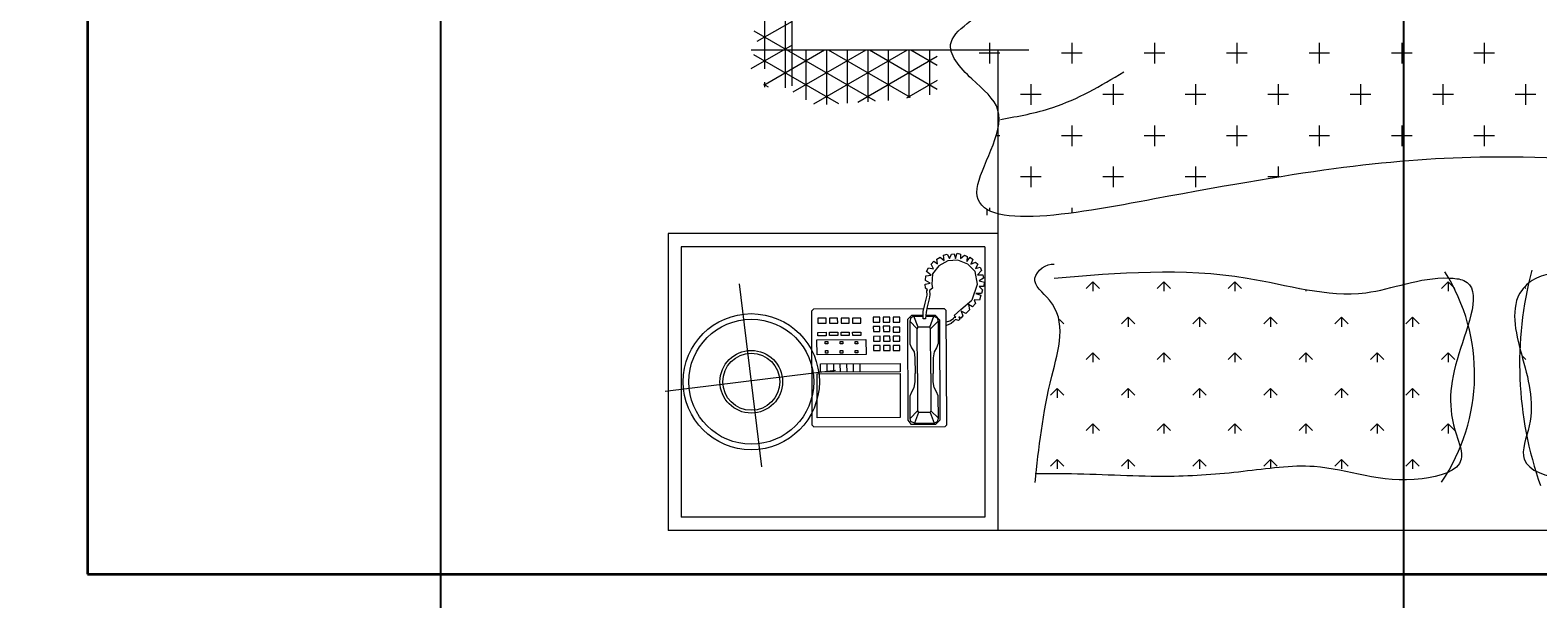
# Model space of a CAD drawing. Units: inches. Extents: x 3731 to 4318, y 1310 to 2388.
# Tile 9 of 57: x 3944 to 4038, y 1363 to 1398. Entities that reach past the tile are written whole.
import ezdxf

# ---------------------------------------------------------------- set-up
doc = ezdxf.new("R2010")
doc.units = ezdxf.units.IN
for name, color, linetype, lineweight in [('A-ANNO-DIMS', 2, 'Continuous', 18), ('A-FURN', 8, 'Continuous', 13), ('A-WALL', 7, 'Continuous', 35)]:
    doc.layers.add(name, color=color, linetype=linetype, lineweight=lineweight)
doc.styles.get("Standard").update_dxf_attribs({"font": 'arial.ttf'})
doc.dimstyles.get("Standard").update_dxf_attribs({"dimtxt": 0.18, "dimasz": 0.18, "dimexe": 0.18, "dimexo": 0.0625, "dimgap": 0.09, "dimtad": 0, "dimtih": 1, "dimtoh": 1, "dimdec": 4, "dimzin": 0, "dimdsep": 46, "dimtxsty": 'Standard', "dimcen": 0.09, "dimadec": 0, "dimazin": 0, "dimtfac": 1, "dimtdec": 4, "dimtofl": 0, "dimtmove": 0, "dimatfit": 3, "dimfxl": 1, "dimtolj": 1, "dimtzin": 0, "dimarcsym": 0})

# ---------------------------------------------------------------- blocks, each defined once
blk = doc.blocks.new('A$C200C7901')
for p, q in [((0.5, 2.3334), (2, 2.3334)), ((2, 2.3334), (2.5, 2.3334)), ((2, 1.6055), (2, 2.3334)), ((2.5, 1.8834), (2.5, 2.3334)), ((1.3176, 2.1721), (1.3075, 2.1822)), ((1.3176, 2.1721), (1.3075, 2.1822)), ((1.206, 2.0681), (1.1997, 2.0744)), ((1.206, 2.0681), (1.1997, 2.0744)), ((1.2019, 1.9645), (1.1997, 1.9666)), ((1.2019, 1.9645), (1.1997, 1.9666)), ((2, 1.8834), (2.5, 1.8834)), ((2.0171, 1.8467), (2.0171, 1.8556)), ((2.0171, 1.8467), (2.0171, 1.8556)), ((2.0129, 1.8445), (2.0129, 1.849)), ((2.0129, 1.8445), (2.0129, 1.849)), ((1.9972, 1.7352), (2.0027, 1.7352)), ((1.9972, 1.7352), (2.0027, 1.7352)), ((2, 1.6963), (2, 1.7248)), ((2, 1.6963), (2, 1.7248)), ((2.3121, 1.6596), (2.3121, 0.0201)), ((1.9533, 1.6055), (2.3741, 1.6055)), ((1.9533, 1.6055), (2.3741, 1.6055))]:
    blk.add_line(p, q)
at = {"linetype": 'ByBlock'}
for p, q in [((2.02, 2.3134), (2.48, 2.3134)), ((2.02, 1.9034), (2.02, 2.3134)), ((2.48, 1.9034), (2.48, 2.3134)), ((1.3714, 2.2259), (1.3714, 2.2402)), ((1.3714, 2.2259), (1.3714, 2.2402)), ((1.4792, 2.2259), (1.4792, 2.2402)), ((1.4792, 2.2259), (1.4792, 2.2402)), ((1.6947, 2.2259), (1.6947, 2.2402)), ((1.6947, 2.2259), (1.6947, 2.2402)), ((1.8025, 2.2259), (1.8025, 2.2402)), ((1.8025, 2.2259), (1.8025, 2.2402)), ((1.9103, 2.2259), (1.9103, 2.2402)), ((1.9103, 2.2259), (1.9103, 2.2402)), ((1.3714, 2.2259), (1.3613, 2.236)), ((1.3714, 2.2259), (1.3613, 2.236)), ((1.3714, 2.2259), (1.3815, 2.236)), ((1.3714, 2.2259), (1.3815, 2.236)), ((1.4792, 2.2259), (1.4691, 2.236)), ((1.4792, 2.2259), (1.4691, 2.236)), ((1.4792, 2.2259), (1.4893, 2.236)), ((1.4792, 2.2259), (1.4893, 2.236)), ((1.587, 2.2259), (1.5769, 2.236)), ((1.587, 2.2259), (1.5769, 2.236)), ((1.587, 2.2259), (1.587, 2.2393)), ((1.587, 2.2259), (1.587, 2.2393)), ((1.587, 2.2259), (1.5971, 2.236)), ((1.587, 2.2259), (1.5971, 2.236)), ((1.6947, 2.2259), (1.6846, 2.236)), ((1.6947, 2.2259), (1.6846, 2.236)), ((1.6947, 2.2259), (1.7048, 2.236)), ((1.6947, 2.2259), (1.7048, 2.236)), ((1.8025, 2.2259), (1.7924, 2.236)), ((1.8025, 2.2259), (1.7924, 2.236)), ((1.8025, 2.2259), (1.8126, 2.236)), ((1.8025, 2.2259), (1.8126, 2.236)), ((1.9103, 2.2259), (1.9002, 2.236)), ((1.9103, 2.2259), (1.9002, 2.236)), ((1.9103, 2.2259), (1.9204, 2.236)), ((1.9103, 2.2259), (1.9204, 2.236)), ((2.3581, 2.2373), (2.3919, 1.9595)), ((1.3176, 2.172), (1.3176, 2.1863)), ((1.3176, 2.172), (1.3176, 2.1863)), ((1.3176, 2.1721), (1.3277, 2.1822)), ((1.3176, 2.1721), (1.3277, 2.1822)), ((1.4253, 2.1721), (1.4152, 2.1822)), ((1.4253, 2.1721), (1.4152, 2.1822)), ((1.4253, 2.172), (1.4253, 2.1863)), ((1.4253, 2.172), (1.4253, 2.1863)), ((1.4253, 2.1721), (1.4354, 2.1822)), ((1.4253, 2.1721), (1.4354, 2.1822)), ((1.5331, 2.1721), (1.523, 2.1822)), ((1.5331, 2.1721), (1.523, 2.1822)), ((1.5331, 2.172), (1.5331, 2.1863)), ((1.5331, 2.172), (1.5331, 2.1863)), ((1.5331, 2.1721), (1.5432, 2.1822)), ((1.5331, 2.1721), (1.5432, 2.1822)), ((1.6409, 2.1721), (1.6308, 2.1822)), ((1.6409, 2.1721), (1.6308, 2.1822)), ((1.6408, 2.172), (1.6408, 2.1863)), ((1.6408, 2.172), (1.6408, 2.1863)), ((1.6409, 2.1721), (1.651, 2.1822)), ((1.6409, 2.1721), (1.651, 2.1822)), ((1.7486, 2.1721), (1.7385, 2.1822)), ((1.7486, 2.1721), (1.7385, 2.1822)), ((1.7486, 2.172), (1.7486, 2.1863)), ((1.7486, 2.172), (1.7486, 2.1863)), ((1.7486, 2.1721), (1.7587, 2.1822)), ((1.7486, 2.1721), (1.7587, 2.1822)), ((1.8564, 2.1721), (1.8463, 2.1822)), ((1.8564, 2.1721), (1.8463, 2.1822)), ((1.8564, 2.172), (1.8564, 2.1863)), ((1.8564, 2.172), (1.8564, 2.1863)), ((1.8564, 2.1721), (1.8665, 2.1822)), ((1.8564, 2.1721), (1.8665, 2.1822)), ((2.0802, 2.176), (2.0777, 2.1734)), ((2.0777, 2.1734), (2.0783, 1.9999)), ((2.2789, 2.1766), (2.0802, 2.176)), ((2.0941, 2.1722), (2.0878, 2.1659)), ((2.1318, 2.1724), (2.0941, 2.1722)), ((2.1267, 2.1711), (2.0966, 2.171)), ((2.1205, 2.1547), (2.1267, 2.1711)), ((2.1267, 2.1711), (2.1318, 2.1686)), ((2.1368, 2.1661), (2.1318, 2.1724)), ((2.2789, 2.1766), (2.2814, 2.1741)), ((2.2814, 2.1741), (2.282, 2.0006)), ((2.0878, 2.1659), (2.0883, 2.015)), ((2.0915, 2.1685), (2.0903, 2.1634)), ((2.0903, 2.1634), (2.1017, 2.1521)), ((2.0903, 2.1634), (2.0904, 2.1295)), ((2.0966, 2.171), (2.0915, 2.1685)), ((2.1029, 2.1547), (2.0966, 2.171)), ((2.1017, 2.1521), (2.1029, 2.1547)), ((2.1019, 2.0956), (2.1017, 2.1521)), ((2.1029, 2.1547), (2.1205, 2.1547)), ((2.1218, 2.1522), (2.1205, 2.1547)), ((2.1331, 2.1636), (2.1218, 2.1522)), ((2.122, 2.0956), (2.1218, 2.1522)), ((2.1318, 2.1686), (2.1331, 2.1636)), ((2.1331, 2.1636), (2.1332, 2.1296)), ((2.1373, 2.014), (2.1368, 2.1661)), ((2.1481, 2.1624), (2.2739, 2.1628)), ((2.1484, 2.0957), (2.1481, 2.1624)), ((2.2739, 2.1628), (2.2741, 2.0961)), ((1.3714, 2.1182), (1.3613, 2.1283)), ((1.3714, 2.1182), (1.3613, 2.1283)), ((1.3714, 2.1182), (1.3714, 2.1325)), ((1.3714, 2.1182), (1.3714, 2.1325)), ((1.3714, 2.1182), (1.3815, 2.1283)), ((1.3714, 2.1182), (1.3815, 2.1283)), ((1.4792, 2.1182), (1.4691, 2.1283)), ((1.4792, 2.1182), (1.4691, 2.1283)), ((1.4792, 2.1182), (1.4792, 2.1325)), ((1.4792, 2.1182), (1.4792, 2.1325)), ((1.4792, 2.1182), (1.4893, 2.1283)), ((1.4792, 2.1182), (1.4893, 2.1283)), ((1.587, 2.1182), (1.5769, 2.1283)), ((1.587, 2.1182), (1.5769, 2.1283)), ((1.587, 2.1182), (1.587, 2.1325)), ((1.587, 2.1182), (1.587, 2.1325)), ((1.587, 2.1182), (1.5971, 2.1283)), ((1.587, 2.1182), (1.5971, 2.1283)), ((1.6947, 2.1182), (1.6846, 2.1283)), ((1.6947, 2.1182), (1.6846, 2.1283)), ((1.6947, 2.1182), (1.6947, 2.1325)), ((1.6947, 2.1182), (1.6947, 2.1325)), ((1.6947, 2.1182), (1.7048, 2.1283)), ((1.6947, 2.1182), (1.7048, 2.1283)), ((1.8025, 2.1182), (1.7924, 2.1283)), ((1.8025, 2.1182), (1.7924, 2.1283)), ((1.8025, 2.1182), (1.8025, 2.1325)), ((1.8025, 2.1182), (1.8025, 2.1325)), ((1.8025, 2.1182), (1.8126, 2.1283)), ((1.8025, 2.1182), (1.8126, 2.1283)), ((1.9103, 2.1182), (1.9002, 2.1283)), ((1.9103, 2.1182), (1.9002, 2.1283)), ((1.9103, 2.1182), (1.9103, 2.1325)), ((1.9103, 2.1182), (1.9103, 2.1325)), ((1.9103, 2.1182), (1.9204, 2.1283)), ((1.9103, 2.1182), (1.9204, 2.1283)), ((2.0904, 2.1295), (2.093, 2.1232)), ((2.1332, 2.1296), (2.1307, 2.1233)), ((2.093, 2.1232), (2.0968, 2.1169)), ((2.0968, 2.1169), (2.098, 2.1081)), ((2.098, 2.1081), (2.0981, 2.0956)), ((2.1269, 2.117), (2.1257, 2.1082)), ((2.1257, 2.1082), (2.1257, 2.0956)), ((2.1307, 2.1233), (2.1269, 2.117)), ((2.2464, 2.0911), (2.5044, 2.1228)), ((2.0982, 2.0717), (2.0981, 2.0956)), ((2.1019, 2.0956), (2.1021, 2.0277)), ((2.122, 2.0956), (2.1222, 2.0277)), ((2.1258, 2.0718), (2.1257, 2.0956)), ((2.2741, 2.0961), (2.1484, 2.0957)), ((2.1484, 2.0932), (2.2691, 2.0936)), ((2.1484, 2.0806), (2.1484, 2.0932)), ((2.2691, 2.081), (2.1484, 2.0806)), ((2.2087, 2.0934), (2.2088, 2.0808)), ((2.2188, 2.0934), (2.2188, 2.0809)), ((2.2288, 2.0935), (2.2289, 2.0809)), ((2.2389, 2.0935), (2.239, 2.0809)), ((2.249, 2.0935), (2.249, 2.081)), ((2.259, 2.0936), (2.2591, 2.081)), ((2.2691, 2.0936), (2.2691, 2.081)), ((1.3176, 2.0643), (1.3075, 2.0744)), ((1.3176, 2.0643), (1.3075, 2.0744)), ((1.3176, 2.0643), (1.3176, 2.0786)), ((1.3176, 2.0643), (1.3176, 2.0786)), ((1.3176, 2.0643), (1.3277, 2.0744)), ((1.3176, 2.0643), (1.3277, 2.0744)), ((1.4253, 2.0643), (1.4152, 2.0744)), ((1.4253, 2.0643), (1.4152, 2.0744)), ((1.4253, 2.0643), (1.4253, 2.0786)), ((1.4253, 2.0643), (1.4253, 2.0786)), ((1.4253, 2.0643), (1.4354, 2.0744)), ((1.4253, 2.0643), (1.4354, 2.0744)), ((1.5331, 2.0643), (1.523, 2.0744)), ((1.5331, 2.0643), (1.523, 2.0744)), ((1.5331, 2.0643), (1.5331, 2.0786)), ((1.5331, 2.0643), (1.5331, 2.0786)), ((1.5331, 2.0643), (1.5432, 2.0744)), ((1.5331, 2.0643), (1.5432, 2.0744)), ((1.6409, 2.0643), (1.6308, 2.0744)), ((1.6409, 2.0643), (1.6308, 2.0744)), ((1.6408, 2.0643), (1.6408, 2.0786)), ((1.6408, 2.0643), (1.6408, 2.0786)), ((1.6409, 2.0643), (1.651, 2.0744)), ((1.6409, 2.0643), (1.651, 2.0744)), ((1.7486, 2.0643), (1.7385, 2.0744)), ((1.7486, 2.0643), (1.7385, 2.0744)), ((1.7486, 2.0643), (1.7486, 2.0786)), ((1.7486, 2.0643), (1.7486, 2.0786)), ((1.7486, 2.0643), (1.7587, 2.0744)), ((1.7486, 2.0643), (1.7587, 2.0744)), ((1.8564, 2.0643), (1.8463, 2.0744)), ((1.8564, 2.0643), (1.8463, 2.0744)), ((1.8564, 2.0643), (1.8564, 2.0786)), ((1.8564, 2.0643), (1.8564, 2.0786)), ((1.8564, 2.0643), (1.8665, 2.0744)), ((1.8564, 2.0643), (1.8665, 2.0744)), ((2.0932, 2.0566), (2.0969, 2.0629)), ((2.0969, 2.0629), (2.0982, 2.0717)), ((2.1271, 2.063), (2.1258, 2.0718)), ((2.1309, 2.0567), (2.1271, 2.063)), ((2.1586, 2.0606), (2.1485, 2.0605)), ((2.1485, 2.0605), (2.1485, 2.053)), ((2.1586, 2.053), (2.1586, 2.0606)), ((2.1636, 2.0606), (2.1636, 2.053)), ((2.1736, 2.0606), (2.1636, 2.0606)), ((2.1737, 2.0531), (2.1736, 2.0606)), ((2.1887, 2.0607), (2.1787, 2.0606)), ((2.1787, 2.0606), (2.1787, 2.0531)), ((2.1888, 2.0531), (2.1887, 2.0607)), ((2.2, 2.067), (2.2742, 2.0672)), ((2.2001, 2.0443), (2.2, 2.067)), ((2.2126, 2.0645), (2.2164, 2.0645)), ((2.2126, 2.0607), (2.2126, 2.0645)), ((2.2164, 2.0607), (2.2126, 2.0607)), ((2.2164, 2.0645), (2.2164, 2.0607)), ((2.2352, 2.0646), (2.239, 2.0646)), ((2.2352, 2.0608), (2.2352, 2.0646)), ((2.239, 2.0608), (2.2352, 2.0608)), ((2.239, 2.0646), (2.239, 2.0608)), ((2.2579, 2.0609), (2.2579, 2.0647)), ((2.2579, 2.0647), (2.2616, 2.0647)), ((2.2616, 2.0609), (2.2579, 2.0609)), ((2.2616, 2.0647), (2.2616, 2.0609)), ((2.2742, 2.0672), (2.2743, 2.0446)), ((2.0907, 2.0503), (2.0932, 2.0566)), ((2.0908, 2.0163), (2.0907, 2.0503)), ((2.1334, 2.0504), (2.1309, 2.0567)), ((2.1336, 2.0165), (2.1334, 2.0504)), ((2.1485, 2.053), (2.1586, 2.053)), ((2.1485, 2.0467), (2.1486, 2.0391)), ((2.1586, 2.0467), (2.1485, 2.0467)), ((2.1486, 2.0391), (2.1586, 2.0392)), ((2.1586, 2.0392), (2.1586, 2.0467)), ((2.1636, 2.053), (2.1737, 2.0531)), ((2.1737, 2.0468), (2.1636, 2.0467)), ((2.1636, 2.0467), (2.1637, 2.0392)), ((2.1637, 2.0392), (2.1737, 2.0392)), ((2.1737, 2.0392), (2.1737, 2.0468)), ((2.1787, 2.0531), (2.1888, 2.0531)), ((2.1787, 2.0468), (2.1787, 2.0392)), ((2.1888, 2.0468), (2.1787, 2.0468)), ((2.1787, 2.0392), (2.1888, 2.0393)), ((2.1888, 2.0393), (2.1888, 2.0468)), ((2.2743, 2.0446), (2.2001, 2.0443)), ((2.2077, 2.0331), (2.2077, 2.0381)), ((2.2077, 2.0381), (2.2202, 2.0381)), ((2.2126, 2.0507), (2.2164, 2.0507)), ((2.2127, 2.0469), (2.2126, 2.0507)), ((2.2164, 2.0469), (2.2127, 2.0469)), ((2.2164, 2.0507), (2.2164, 2.0469)), ((2.2202, 2.0381), (2.2203, 2.0331)), ((2.2253, 2.0381), (2.2378, 2.0382)), ((2.2253, 2.0331), (2.2253, 2.0381)), ((2.2353, 2.0508), (2.2391, 2.0508)), ((2.2353, 2.047), (2.2353, 2.0508)), ((2.2391, 2.047), (2.2353, 2.047)), ((2.2378, 2.0382), (2.2379, 2.0332)), ((2.2391, 2.0508), (2.2391, 2.047)), ((2.2429, 2.0332), (2.2429, 2.0382)), ((2.2429, 2.0382), (2.2554, 2.0382)), ((2.2554, 2.0382), (2.2555, 2.0332)), ((2.2579, 2.0508), (2.2617, 2.0508)), ((2.2579, 2.0471), (2.2579, 2.0508)), ((2.2617, 2.0471), (2.2579, 2.0471)), ((2.2605, 2.0332), (2.2605, 2.0383)), ((2.2605, 2.0383), (2.273, 2.0383)), ((2.2617, 2.0508), (2.2617, 2.0471)), ((2.273, 2.0383), (2.2731, 2.0333)), ((1.3714, 2.0104), (1.3613, 2.0205)), ((1.3714, 2.0104), (1.3613, 2.0205)), ((1.3714, 2.0104), (1.3714, 2.0247)), ((1.3714, 2.0104), (1.3714, 2.0247)), ((1.3714, 2.0104), (1.3815, 2.0205)), ((1.3714, 2.0104), (1.3815, 2.0205)), ((1.4792, 2.0104), (1.4691, 2.0205)), ((1.4792, 2.0104), (1.4691, 2.0205)), ((1.4792, 2.0104), (1.4792, 2.0247)), ((1.4792, 2.0104), (1.4792, 2.0247)), ((1.4792, 2.0104), (1.4893, 2.0205)), ((1.4792, 2.0104), (1.4893, 2.0205)), ((1.587, 2.0104), (1.5769, 2.0205)), ((1.587, 2.0104), (1.5769, 2.0205)), ((1.587, 2.0104), (1.587, 2.0247)), ((1.587, 2.0104), (1.587, 2.0247)), ((1.587, 2.0104), (1.5971, 2.0205)), ((1.587, 2.0104), (1.5971, 2.0205)), ((1.6947, 2.0104), (1.6846, 2.0205)), ((1.6947, 2.0104), (1.6846, 2.0205)), ((1.6947, 2.0104), (1.6947, 2.0247)), ((1.6947, 2.0104), (1.6947, 2.0247)), ((1.6947, 2.0104), (1.7048, 2.0205)), ((1.6947, 2.0104), (1.7048, 2.0205)), ((1.8025, 2.0104), (1.7924, 2.0205)), ((1.8025, 2.0104), (1.7924, 2.0205)), ((1.8025, 2.0104), (1.8025, 2.0247)), ((1.8025, 2.0104), (1.8025, 2.0247)), ((1.8025, 2.0104), (1.8126, 2.0205)), ((1.8025, 2.0104), (1.8126, 2.0205)), ((1.9068, 2.0139), (1.9002, 2.0205)), ((1.9068, 2.0139), (1.9002, 2.0205)), ((2.053, 2.0084), (2.0563, 2.0119)), ((2.0563, 2.0119), (2.0594, 2.0095)), ((2.0576, 2.0133), (2.0598, 2.0155)), ((2.0594, 2.0095), (2.0576, 2.0133)), ((2.0598, 2.0155), (2.0645, 2.0137)), ((2.0645, 2.0137), (2.0671, 2.0162)), ((2.0676, 2.012), (2.0663, 2.0102)), ((2.0671, 2.0162), (2.0707, 2.0197)), ((2.0727, 2.016), (2.0676, 2.012)), ((2.0707, 2.0197), (2.0782, 2.0226)), ((2.0782, 2.0175), (2.0727, 2.016)), ((2.0883, 2.015), (2.0946, 2.0075)), ((2.0908, 2.0163), (2.1021, 2.0277)), ((2.0921, 2.0113), (2.0908, 2.0163)), ((2.0971, 2.0088), (2.0921, 2.0113)), ((2.1034, 2.0252), (2.0971, 2.0088)), ((2.1021, 2.0277), (2.1034, 2.0252)), ((2.1034, 2.0252), (2.121, 2.0252)), ((2.109, 2.0025), (2.1097, 2.0126)), ((2.1097, 2.0126), (2.1135, 2.0126)), ((2.1135, 2.0126), (2.1133, 2.0018)), ((2.1222, 2.0277), (2.121, 2.0252)), ((2.121, 2.0252), (2.1273, 2.0089)), ((2.1336, 2.0165), (2.1222, 2.0277)), ((2.1273, 2.0089), (2.1323, 2.0114)), ((2.1311, 2.0077), (2.1373, 2.014)), ((2.1323, 2.0114), (2.1336, 2.0165)), ((2.1586, 2.0329), (2.1486, 2.0329)), ((2.1486, 2.0329), (2.1486, 2.0253)), ((2.1486, 2.0253), (2.1587, 2.0253)), ((2.1587, 2.0178), (2.1486, 2.0178)), ((2.1486, 2.0178), (2.1487, 2.0102)), ((2.1587, 2.0253), (2.1586, 2.0329)), ((2.1587, 2.0103), (2.1587, 2.0178)), ((2.1637, 2.0317), (2.1637, 2.0241)), ((2.1737, 2.0317), (2.1637, 2.0317)), ((2.1637, 2.0241), (2.1738, 2.0241)), ((2.1738, 2.0179), (2.1637, 2.0178)), ((2.1637, 2.0178), (2.1638, 2.0103)), ((2.1738, 2.0241), (2.1737, 2.0317)), ((2.1738, 2.0103), (2.1738, 2.0179)), ((2.1788, 2.0317), (2.1788, 2.0242)), ((2.1888, 2.0317), (2.1788, 2.0317)), ((2.1788, 2.0242), (2.1889, 2.0242)), ((2.1788, 2.0179), (2.1788, 2.0103)), ((2.1889, 2.0179), (2.1788, 2.0179)), ((2.1889, 2.0242), (2.1888, 2.0317)), ((2.1889, 2.0104), (2.1889, 2.0179)), ((2.2203, 2.0331), (2.2077, 2.0331)), ((2.2203, 2.0193), (2.2077, 2.0192)), ((2.2077, 2.0192), (2.2078, 2.0117)), ((2.2078, 2.0117), (2.2203, 2.0117)), ((2.2203, 2.0117), (2.2203, 2.0193)), ((2.2379, 2.0332), (2.2253, 2.0331)), ((2.2379, 2.0193), (2.2253, 2.0193)), ((2.2253, 2.0193), (2.2254, 2.0117)), ((2.2254, 2.0117), (2.2379, 2.0118)), ((2.2379, 2.0118), (2.2379, 2.0193)), ((2.2555, 2.0332), (2.2429, 2.0332)), ((2.2555, 2.0194), (2.2429, 2.0193)), ((2.2429, 2.0193), (2.243, 2.0118)), ((2.243, 2.0118), (2.2555, 2.0118)), ((2.2555, 2.0118), (2.2555, 2.0194)), ((2.2731, 2.0333), (2.2605, 2.0332)), ((2.2605, 2.0194), (2.2606, 2.0119)), ((2.2731, 2.0194), (2.2605, 2.0194)), ((2.2606, 2.0119), (2.2731, 2.0119)), ((2.2731, 2.0119), (2.2731, 2.0194)), ((2.0338, 1.9895), (2.0386, 1.9946)), ((2.0358, 1.9839), (2.0338, 1.9895)), ((2.0386, 1.9946), (2.0444, 1.9911)), ((2.0561, 1.9986), (2.0396, 1.9844)), ((2.0431, 1.999), (2.0488, 2.0046)), ((2.0444, 1.9911), (2.0431, 1.999)), ((2.0488, 2.0046), (2.0557, 2.0011)), ((2.0557, 2.0011), (2.053, 2.0084)), ((2.0663, 2.0077), (2.0561, 1.9986)), ((2.0663, 2.0102), (2.0636, 2.0104)), ((2.0636, 2.0104), (2.0663, 2.0077)), ((2.0783, 1.9999), (2.0808, 1.9974)), ((2.0808, 1.9974), (2.1079, 1.9975)), ((2.0946, 2.0075), (2.1093, 2.0076)), ((2.1094, 2.0088), (2.0971, 2.0088)), ((2.1042, 1.9824), (2.1072, 1.9944)), ((2.1072, 1.9944), (2.109, 2.0025)), ((2.1103, 1.989), (2.1073, 1.9771)), ((2.1133, 2.0018), (2.1103, 1.989)), ((2.1123, 1.9975), (2.2795, 1.9981)), ((2.1273, 2.0089), (2.1134, 2.0088)), ((2.1134, 2.0076), (2.1311, 2.0077)), ((2.1487, 2.0102), (2.1587, 2.0103)), ((2.1638, 2.0103), (2.1738, 2.0103)), ((2.1788, 2.0103), (2.1889, 2.0104)), ((2.282, 2.0006), (2.2795, 1.9981)), ((1.3176, 1.9565), (1.3075, 1.9666)), ((1.3176, 1.9565), (1.3075, 1.9666)), ((1.3176, 1.9565), (1.3176, 1.9708)), ((1.3176, 1.9565), (1.3176, 1.9708)), ((1.3176, 1.9565), (1.3277, 1.9666)), ((1.3176, 1.9565), (1.3277, 1.9666)), ((1.4253, 1.9703), (1.4253, 1.9708)), ((1.4253, 1.9703), (1.4253, 1.9708)), ((1.5331, 1.9683), (1.5331, 1.9708)), ((1.5331, 1.9683), (1.5331, 1.9708)), ((1.543, 1.9665), (1.5432, 1.9666)), ((1.543, 1.9665), (1.5432, 1.9666)), ((1.6409, 1.9565), (1.6308, 1.9666)), ((1.6409, 1.9565), (1.6308, 1.9666)), ((1.6408, 1.9565), (1.6408, 1.9708)), ((1.6408, 1.9565), (1.6408, 1.9708)), ((1.6409, 1.9565), (1.651, 1.9666)), ((1.6409, 1.9565), (1.651, 1.9666)), ((1.7486, 1.9565), (1.7385, 1.9666)), ((1.7486, 1.9565), (1.7385, 1.9666)), ((1.7486, 1.9565), (1.7486, 1.9708)), ((1.7486, 1.9565), (1.7486, 1.9708)), ((1.7486, 1.9565), (1.7587, 1.9666)), ((1.7486, 1.9565), (1.7587, 1.9666)), ((1.8564, 1.9565), (1.8463, 1.9666)), ((1.8564, 1.9565), (1.8463, 1.9666)), ((1.8564, 1.9565), (1.8564, 1.9708)), ((1.8564, 1.9565), (1.8564, 1.9708)), ((1.8564, 1.9565), (1.8665, 1.9666)), ((1.8564, 1.9565), (1.8665, 1.9666)), ((2.0234, 1.9686), (2.0251, 1.9745)), ((2.0287, 1.9636), (2.0234, 1.9686)), ((2.0251, 1.9745), (2.0333, 1.9743)), ((2.0259, 1.977), (2.0281, 1.9847)), ((2.0333, 1.9743), (2.0259, 1.977)), ((2.0281, 1.9847), (2.0358, 1.9839)), ((2.0393, 1.984), (2.031, 1.96)), ((2.0992, 1.9663), (2.1038, 1.9697)), ((2.1002, 1.9605), (2.0992, 1.9663)), ((2.1035, 1.9763), (2.1042, 1.9824)), ((2.1038, 1.9697), (2.1035, 1.9763)), ((2.1076, 1.9704), (2.1068, 1.9689)), ((2.1068, 1.9689), (2.1096, 1.9661)), ((2.1073, 1.9771), (2.1076, 1.9704)), ((2.1096, 1.9661), (2.1101, 1.96)), ((2.0206, 1.9572), (2.0218, 1.9635)), ((2.0285, 1.9549), (2.0206, 1.9572)), ((2.0218, 1.9635), (2.0287, 1.9636)), ((2.0219, 1.9511), (2.0285, 1.9549)), ((2.0229, 1.946), (2.0219, 1.9511)), ((2.0308, 1.9462), (2.0229, 1.946)), ((2.0247, 1.9394), (2.0308, 1.9462)), ((2.031, 1.96), (2.0346, 1.9409)), ((2.0894, 1.9322), (2.099, 1.9444)), ((2.099, 1.9444), (2.1002, 1.9605)), ((2.1094, 1.9475), (2.1013, 1.9467)), ((2.1013, 1.9467), (2.1084, 1.9412)), ((2.1101, 1.96), (2.1028, 1.9587)), ((2.1028, 1.9587), (2.1099, 1.9544)), ((2.1099, 1.9544), (2.1094, 1.9475)), ((2.0268, 1.9343), (2.0247, 1.9394)), ((2.0341, 1.9366), (2.0268, 1.9343)), ((2.0306, 1.9297), (2.0341, 1.9366)), ((2.0339, 1.9267), (2.0306, 1.9297)), ((2.041, 1.9297), (2.0339, 1.9267)), ((2.0346, 1.9409), (2.0459, 1.93)), ((2.038, 1.9228), (2.041, 1.9297)), ((2.0421, 1.9193), (2.038, 1.9228)), ((2.0474, 1.9259), (2.0421, 1.9193)), ((2.0459, 1.93), (2.0607, 1.9237)), ((2.0467, 1.9183), (2.0474, 1.9259)), ((2.0566, 1.9214), (2.0508, 1.9163)), ((2.0569, 1.9145), (2.0566, 1.9214)), ((2.0607, 1.9237), (2.0759, 1.925)), ((2.0645, 1.9214), (2.0617, 1.9133)), ((2.0663, 1.914), (2.0645, 1.9214)), ((2.0736, 1.9214), (2.0706, 1.9146)), ((2.077, 1.9146), (2.0736, 1.9214)), ((2.0759, 1.925), (2.0894, 1.9322)), ((2.0876, 1.9195), (2.0815, 1.9245)), ((2.0815, 1.9245), (2.0823, 1.9161)), ((2.0925, 1.9225), (2.0876, 1.9195)), ((2.0973, 1.9251), (2.0914, 1.9294)), ((2.0914, 1.9294), (2.0925, 1.9225)), ((2.1011, 1.9297), (2.0973, 1.9251)), ((2.1051, 1.9353), (2.0975, 1.9368)), ((2.0975, 1.9368), (2.1011, 1.9297)), ((2.1084, 1.9412), (2.1051, 1.9353)), ((2.02, 1.9034), (2.48, 1.9034)), ((2.0508, 1.9163), (2.0467, 1.9183)), ((2.0617, 1.9133), (2.0569, 1.9145)), ((2.0706, 1.9146), (2.0663, 1.914)), ((2.0823, 1.9161), (2.077, 1.9146)), ((1.8879, 1.8445), (1.8879, 1.8523)), ((1.8879, 1.8445), (1.8879, 1.8523)), ((1.7004, 1.782), (1.7004, 1.8133)), ((1.7004, 1.782), (1.7004, 1.8133)), ((1.8254, 1.782), (1.8254, 1.8133)), ((1.8254, 1.782), (1.8254, 1.8133)), ((1.9504, 1.782), (1.9504, 1.8133)), ((1.9504, 1.782), (1.9504, 1.8133)), ((1.573, 1.7977), (1.591, 1.7977)), ((1.573, 1.7977), (1.591, 1.7977)), ((1.5754, 1.782), (1.5754, 1.7981)), ((1.5754, 1.782), (1.5754, 1.7981)), ((1.6847, 1.7977), (1.716, 1.7977)), ((1.6847, 1.7977), (1.716, 1.7977)), ((1.8097, 1.7977), (1.841, 1.7977)), ((1.8097, 1.7977), (1.841, 1.7977)), ((1.9347, 1.7977), (1.966, 1.7977)), ((1.9347, 1.7977), (1.966, 1.7977)), ((1.2629, 1.7195), (1.2629, 1.7508)), ((1.2629, 1.7195), (1.2629, 1.7508)), ((1.3879, 1.7195), (1.3879, 1.7508)), ((1.3879, 1.7195), (1.3879, 1.7508)), ((1.5129, 1.7195), (1.5129, 1.7508)), ((1.5129, 1.7195), (1.5129, 1.7508)), ((1.6379, 1.7195), (1.6379, 1.7508)), ((1.6379, 1.7195), (1.6379, 1.7508)), ((1.7629, 1.7195), (1.7629, 1.7508)), ((1.7629, 1.7195), (1.7629, 1.7508)), ((1.8879, 1.7195), (1.8879, 1.7508)), ((1.8879, 1.7195), (1.8879, 1.7508)), ((1.2472, 1.7352), (1.2785, 1.7352)), ((1.2472, 1.7352), (1.2785, 1.7352)), ((1.3722, 1.7352), (1.4035, 1.7352)), ((1.3722, 1.7352), (1.4035, 1.7352)), ((1.4972, 1.7352), (1.5285, 1.7352)), ((1.4972, 1.7352), (1.5285, 1.7352)), ((1.6222, 1.7352), (1.6535, 1.7352)), ((1.6222, 1.7352), (1.6535, 1.7352)), ((1.7472, 1.7352), (1.7785, 1.7352)), ((1.7472, 1.7352), (1.7785, 1.7352)), ((1.8722, 1.7352), (1.9035, 1.7352)), ((1.8722, 1.7352), (1.9035, 1.7352)), ((1.1847, 1.6727), (1.216, 1.6727)), ((1.1847, 1.6727), (1.216, 1.6727)), ((1.2004, 1.657), (1.2004, 1.6883)), ((1.2004, 1.657), (1.2004, 1.6883)), ((1.3097, 1.6727), (1.341, 1.6727)), ((1.3097, 1.6727), (1.341, 1.6727)), ((1.3254, 1.657), (1.3254, 1.6883)), ((1.3254, 1.657), (1.3254, 1.6883)), ((1.4347, 1.6727), (1.466, 1.6727)), ((1.4347, 1.6727), (1.466, 1.6727)), ((1.4504, 1.657), (1.4504, 1.6883)), ((1.4504, 1.657), (1.4504, 1.6883)), ((1.5597, 1.6727), (1.591, 1.6727)), ((1.5597, 1.6727), (1.591, 1.6727)), ((1.5754, 1.657), (1.5754, 1.6883)), ((1.5754, 1.657), (1.5754, 1.6883)), ((1.6847, 1.6727), (1.716, 1.6727)), ((1.6847, 1.6727), (1.716, 1.6727)), ((1.7004, 1.657), (1.7004, 1.6883)), ((1.7004, 1.657), (1.7004, 1.6883)), ((1.8097, 1.6727), (1.841, 1.6727)), ((1.8097, 1.6727), (1.841, 1.6727)), ((1.8254, 1.657), (1.8254, 1.6883)), ((1.8254, 1.657), (1.8254, 1.6883)), ((1.9347, 1.6727), (1.966, 1.6727)), ((1.9347, 1.6727), (1.966, 1.6727)), ((1.9504, 1.657), (1.9504, 1.6883)), ((1.9504, 1.657), (1.9504, 1.6883)), ((2.0919, 1.6152), (2.2125, 1.6848)), ((2.0919, 1.6152), (2.2125, 1.6848)), ((2.0919, 1.6513), (2.1386, 1.6782)), ((2.0919, 1.6513), (2.1386, 1.6782)), ((2.1037, 1.6055), (2.1037, 1.673)), ((2.1037, 1.6055), (2.1037, 1.673)), ((2.1327, 1.6773), (2.2571, 1.6055)), ((2.1327, 1.6773), (2.2571, 1.6055)), ((2.1349, 1.6055), (2.1349, 1.6777)), ((2.1349, 1.6055), (2.1349, 1.6777)), ((2.1377, 1.6055), (2.2798, 1.6876)), ((2.1377, 1.6055), (2.2798, 1.6876)), ((2.1662, 1.6055), (2.1662, 1.6817)), ((2.1662, 1.6055), (2.1662, 1.6817)), ((2.1854, 1.683), (2.3697, 1.5766)), ((2.1854, 1.683), (2.3697, 1.5766)), ((2.1974, 1.6055), (2.1974, 1.6838)), ((2.1974, 1.6055), (2.1974, 1.6838)), ((2.2002, 1.6055), (2.3109, 1.6694)), ((2.2002, 1.6055), (2.3109, 1.6694)), ((2.2287, 1.6055), (2.2287, 1.6859)), ((2.2287, 1.6055), (2.2287, 1.6859)), ((2.2414, 1.6868), (2.3699, 1.6126)), ((2.2414, 1.6868), (2.3699, 1.6126)), ((2.2599, 1.6055), (2.2599, 1.688)), ((2.2599, 1.6055), (2.2599, 1.688)), ((2.2912, 1.6055), (2.2912, 1.6809)), ((2.2912, 1.6055), (2.2912, 1.6809)), ((2.0919, 1.6649), (2.1946, 1.6055)), ((2.0919, 1.6649), (2.1946, 1.6055)), ((2.2627, 1.6055), (2.3551, 1.6589)), ((2.2627, 1.6055), (2.3551, 1.6589)), ((2.3224, 0.0468), (2.3224, 1.6627)), ((2.3224, 0.0468), (2.3224, 1.6627)), ((2.3476, 1.6616), (2.3547, 1.6575)), ((2.3476, 1.6616), (2.3547, 1.6575)), ((2.3537, 1.6539), (2.3537, 1.6616)), ((2.3537, 1.6539), (2.3537, 1.6616)), ((1.2629, 1.5945), (1.2629, 1.6258)), ((1.2629, 1.5945), (1.2629, 1.6258)), ((1.3879, 1.5945), (1.3879, 1.6258)), ((1.3879, 1.5945), (1.3879, 1.6258)), ((1.5129, 1.5945), (1.5129, 1.6258)), ((1.5129, 1.5945), (1.5129, 1.6258)), ((1.6379, 1.5945), (1.6379, 1.6258)), ((1.6379, 1.5945), (1.6379, 1.6258)), ((1.7629, 1.5945), (1.7629, 1.6258)), ((1.7629, 1.5945), (1.7629, 1.6258)), ((1.8879, 1.5945), (1.8879, 1.6258)), ((1.8879, 1.5945), (1.8879, 1.6258)), ((2.0129, 1.5945), (2.0129, 1.6258)), ((2.0129, 1.5945), (2.0129, 1.6258)), ((2.0919, 1.6288), (2.1321, 1.6055)), ((2.0919, 1.6288), (2.1321, 1.6055)), ((2.3121, 1.598), (2.3745, 1.634)), ((2.3121, 1.598), (2.3745, 1.634)), ((2.3537, 0.0056), (2.3537, 1.634)), ((2.3537, 0.0056), (2.3537, 1.634)), ((1.2472, 1.6102), (1.2785, 1.6102)), ((1.2472, 1.6102), (1.2785, 1.6102)), ((1.3722, 1.6102), (1.4035, 1.6102)), ((1.3722, 1.6102), (1.4035, 1.6102)), ((1.4972, 1.6102), (1.5285, 1.6102)), ((1.4972, 1.6102), (1.5285, 1.6102)), ((1.6222, 1.6102), (1.6535, 1.6102)), ((1.6222, 1.6102), (1.6535, 1.6102)), ((1.7472, 1.6102), (1.7785, 1.6102)), ((1.7472, 1.6102), (1.7785, 1.6102)), ((1.8722, 1.6102), (1.9035, 1.6102)), ((1.8722, 1.6102), (1.9035, 1.6102)), ((1.9972, 1.6102), (2.0285, 1.6102)), ((1.9972, 1.6102), (2.0285, 1.6102)), ((2.3121, 1.5619), (2.3654, 1.5926)), ((2.3121, 1.5619), (2.3654, 1.5926))]:
    blk.add_line(p, q, dxfattribs=at)
for radius in [0.1032, 0.0947, 0.0475, 0.0432]:
    blk.add_circle((2.3739, 2.1081), radius, dxfattribs=at)
for centre, radius, start, end in [((0.658, 2.0811), 0.5513, 345.0722, 19.5492), ((1.5685, 2.097), 0.291, 145.8603, 212.2445)]:
    blk.add_arc(centre, radius, start, end)
for points, knots in [([(0.5854, 1.951), (0.6835, 1.9407), (0.8425, 1.9242), (1.0374, 2.0054), (1.1564, 1.9255), (1.2274, 1.9841), (1.2052, 2.0751), (1.1815, 2.152), (1.2176, 2.2368), (1.0992, 2.2731), (1.0008, 2.2255), (0.8698, 2.246), (0.7481, 2.2548), (0.6426, 2.2473), (0.5746, 2.2478), (0.5562, 2.2479)], [0, 0, 0, 0, 292.165466, 473.33038, 601.631673, 630.723769, 727.138505, 836.819956, 887.958136, 954.42438, 1118.989809, 1227.016542, 1338.750986, 1487.447361, 1542.751028, 1542.751028, 1542.751028, 1542.751028]), ([(1.9146, 1.951), (1.8174, 1.9428), (1.6601, 1.9297), (1.4574, 1.9942), (1.3549, 1.9462), (1.2593, 1.9563), (1.314, 2.0834), (1.3193, 2.1569), (1.2853, 2.2393), (1.4031, 2.2724), (1.4987, 2.2256), (1.6304, 2.2459), (1.7519, 2.2548), (1.8574, 2.2473), (1.9254, 2.2478), (1.9438, 2.2479)], [0, 0, 0, 0, 292.165466, 473.33038, 601.631673, 624.236147, 735.870502, 858.452188, 896.317728, 962.783971, 1127.3494, 1235.376134, 1347.110578, 1495.806953, 1551.11062, 1551.11062, 1551.11062, 1551.11062]), ([(1.9438, 2.2608), (1.9381, 2.2086), (1.9282, 2.1195), (1.8897, 2.0022), (1.9591, 1.9538), (1.9264, 1.9278), (1.9146, 1.93)], [0, 0, 0, 0, 163.411291, 278.570782, 318.445997, 354.484131, 354.484131, 354.484131, 354.484131]), ([(0.4485, 1.7835), (0.4321, 1.7496), (0.4062, 1.6964), (0.49, 1.6713), (0.4719, 1.5969), (0.4123, 1.592), (0.4233, 1.5337), (0.4954, 1.5086), (0.4012, 1.4738), (0.3253, 1.4306), (0.4113, 1.3764), (0.3688, 1.3065), (0.5579, 1.2663), (0.741, 1.4533), (1.1127, 1.1109), (1.4811, 1.2478), (1.7885, 1.3492), (2.0357, 1.1637), (2.0748, 1.2974), (2.0876, 1.349), (2.0192, 1.3805), (2.0564, 1.4298), (2.0588, 1.4846), (1.9759, 1.5349), (2.1004, 1.5845), (2.0397, 1.6519), (1.971, 1.7053), (2.1104, 1.8981), (1.5946, 1.7967), (1.2448, 1.7472), (0.8129, 1.7935), (0.4953, 1.8548), (0.4582, 1.7983), (0.4485, 1.7835)], [0, 0, 0, 0, 88.420092, 139.08588, 204.302936, 239.695496, 287.801042, 327.365471, 412.960499, 463.626286, 552.059846, 584.668336, 662.614915, 940.993281, 1309.926334, 1844.022653, 1996.276242, 2316.43048, 2341.441004, 2404.707416, 2449.463774, 2514.680778, 2538.40571, 2613.031547, 2697.13096, 2760.903931, 2822.692699, 2945.47, 3215.060018, 3725.584917, 4361.974444, 4504.671998, 4555.32777, 4555.32777, 4555.32777, 4555.32777])]:
    blk.add_open_spline(points, degree=3, knots=knots)
blk.add_open_spline([(1.996, 1.7104), (1.9692, 1.7057), (1.9025, 1.6938), (1.844, 1.6592), (1.809, 1.6385)], degree=3, knots=[0, 0, 0, 0, 81.132613, 201.738644, 201.738644, 201.738644, 201.738644], dxfattribs=at)
blk.add_open_spline([(1.996, 1.7104), (1.9692, 1.7057), (1.9025, 1.6938), (1.844, 1.6592), (1.809, 1.6385)], degree=3, knots=[0, 0, 0, 0, 81.132613, 201.738644, 201.738644, 201.738644, 201.738644], dxfattribs=at)
blk = doc.blocks.new('*D32')
at = {"layer": 'A-ANNO-DIMS', "color": 0, "lineweight": -2, "transparency": 16777216}
for p, q in [((4269.211, 1592.319), (4269.211, 1310.251)), ((3835.209, 1359.319), (3835.209, 1310.251)), ((3835.389, 1310.431), (4051.918, 1310.431)), ((4269.031, 1310.431), (4052.502, 1310.431))]:
    blk.add_line(p, q, dxfattribs=at)
at = {"layer": 'A-ANNO-DIMS', "color": 0, "transparency": 16777216}
for points in [[(3835.389, 1310.461), (3835.389, 1310.401), (3835.209, 1310.431)], [(4269.031, 1310.461), (4269.031, 1310.401), (4269.211, 1310.431)]]:
    blk.add_solid(points, dxfattribs=at)
at = {"layer": 'Defpoints', "color": 0, "transparency": 16777216}
for p in [(4269.211, 1592.382), (3835.209, 1359.382), (4269.211, 1310.431)]:
    blk.add_point(p, dxfattribs=at)
at = {"layer": 'A-ANNO-DIMS', "color": 0, "transparency": 16777216, "insert": (4052.21, 1310.431), "char_height": 0.18, "attachment_point": 5}
blk.add_mtext('\\A1;434', dxfattribs=at)
blk = doc.blocks.new('*D44')
at = {"layer": 'A-ANNO-DIMS', "color": 0, "lineweight": -2, "transparency": 16777216}
for p, q in [((3969.209, 1874.319), (3969.209, 1310.251)), ((4029.209, 1874.319), (4029.209, 1310.251)), ((3969.389, 1310.431), (3998.99, 1310.431)), ((4029.029, 1310.431), (3999.428, 1310.431))]:
    blk.add_line(p, q, dxfattribs=at)
at = {"layer": 'A-ANNO-DIMS', "color": 0, "transparency": 16777216}
for points in [[(3969.389, 1310.461), (3969.389, 1310.401), (3969.209, 1310.431)], [(4029.029, 1310.461), (4029.029, 1310.401), (4029.209, 1310.431)]]:
    blk.add_solid(points, dxfattribs=at)
at = {"layer": 'Defpoints', "color": 0, "transparency": 16777216}
for p in [(3969.209, 1874.382), (4029.209, 1874.382), (4029.209, 1310.431)]:
    blk.add_point(p, dxfattribs=at)
at = {"layer": 'A-ANNO-DIMS', "color": 0, "transparency": 16777216, "insert": (3999.209, 1310.431), "char_height": 0.18, "attachment_point": 5}
blk.add_mtext('\\A1;60', dxfattribs=at)

msp = doc.modelspace()

# ---------------------------------------------------------------- linework, layer by layer
at = {"layer": 'A-WALL'}
for p, q in [((3947.211, 1484.382), (3947.211, 1364.382)), ((3947.211, 1364.382), (4109.211, 1364.382))]:
    msp.add_line(p, q, dxfattribs=at)

# ---------------------------------------------------------------- block references
at = {"layer": 'A-FURN', "xscale": 41.1071563136412, "yscale": 41.1071563136412, "zscale": 41.1071563136412, "rotation": 180}
msp.add_blockref('A$C200C7901', (4086.148, 1463.037), dxfattribs=at)

# ---------------------------------------------------------------- dimensions: what is measured, and where the dimension line sits
at = {"layer": 'A-ANNO-DIMS'}
for base, p1, p2, picture, middle in [((4029.209, 1310.431), (3969.209, 1874.382), (4029.209, 1874.382), '*D44', (3999.209, 1310.431)), ((4269.211, 1310.431), (3835.209, 1359.382), (4269.211, 1592.382), '*D32', (4052.21, 1310.431))]:
    dim = msp.add_linear_dim(base=base, p1=p1, p2=p2, dimstyle='Standard', override={"dimdec": 0, "dimlfac": 1, "dimrnd": 0, "dimzin": 0, "dimdsep": 46, "dimlunit": 2}, dxfattribs=at)
    dim.commit()
    dim.dimension.update_dxf_attribs({"geometry": picture, "text_midpoint": middle})

doc.saveas('drawing.dxf')
